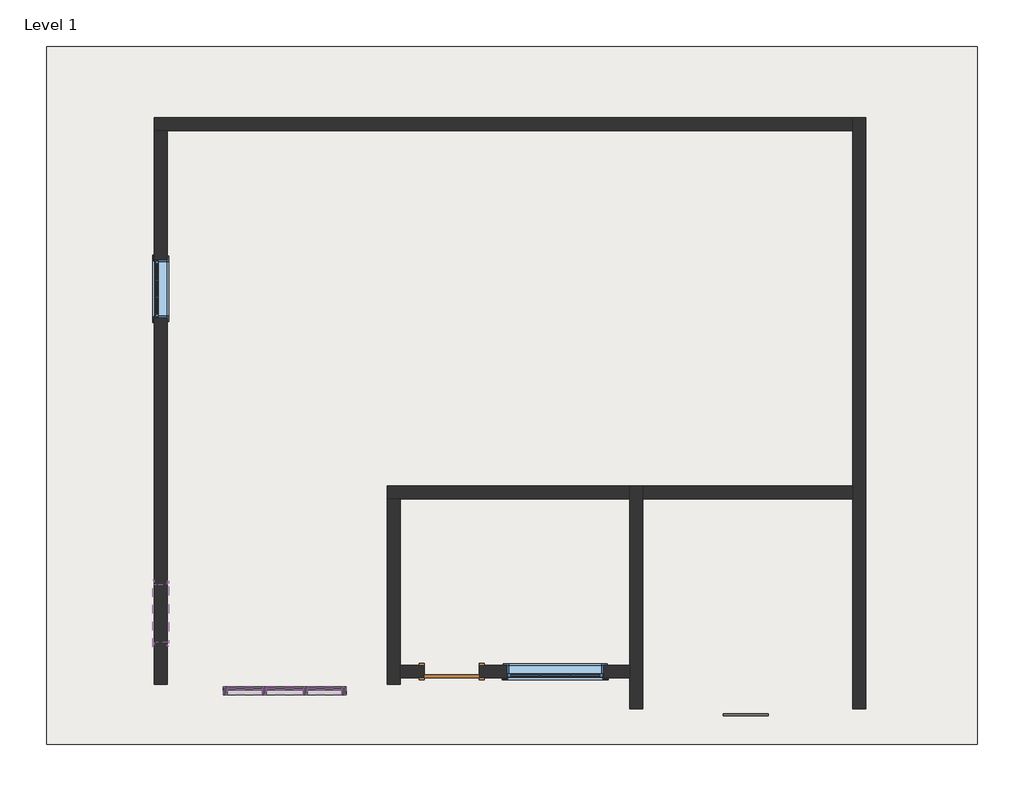
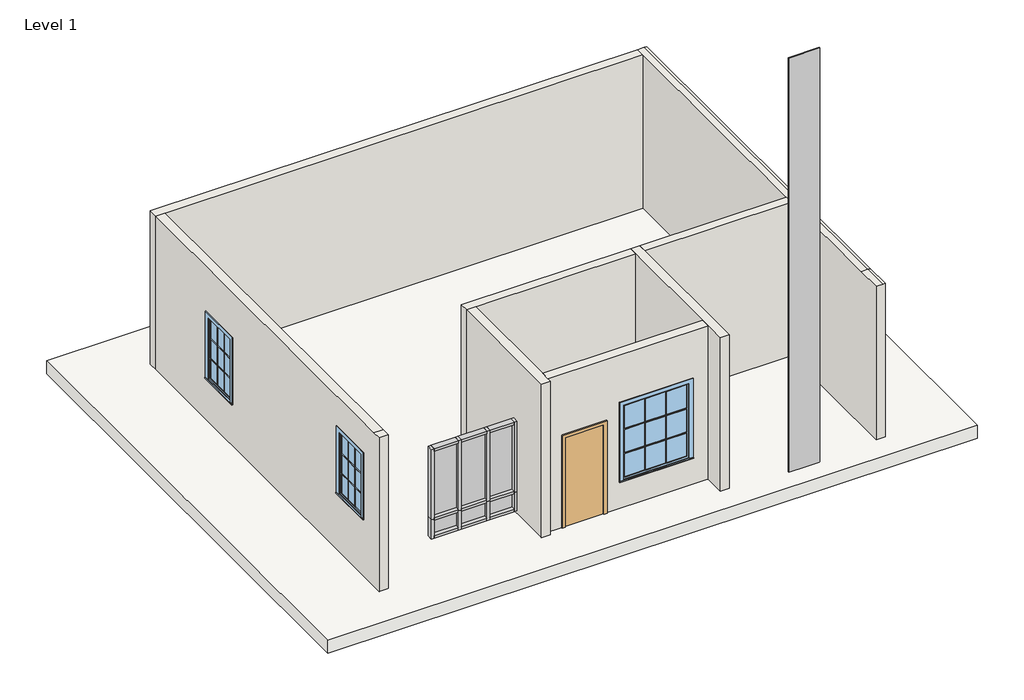
# One storey: 17 members, 8 walls, 7 plates, 3 windows, 1 door, 1 slab.
"""IFC4 building model written with IfcOpenShell, lengths in millimetres."""

from ifc_helpers import new_model, si_unit, frame, origin, origin_with_axes, place, context, project, spatial, polyline, outline, extrude, faceted_brep, transform, mapped, element, save
from components import door_f75d31f8, member_6374d63f, member_ffd4c858, member_912d8bb3, member_c5d18237, member_71656fef, member_15823cb3, member_c78c2eae, member_bdb631d2, system_panel_glazed_05561604, system_panel_glazed_5c6b2ea2, system_panel_glazed_7f181415, system_panel_glazed_51fb9f70, system_panel_glazed_62cbeebf, window_58e1470a, window_f2d3b6b9

model = new_model("IFC4")

# Units and contexts
model_context = context("Model", 3, world=origin())
ifc_project = project(units=[si_unit("LENGTHUNIT", "METRE", prefix="MILLI")], contexts=[model_context])

# Site, building, storey
site = spatial("IfcSite", under=ifc_project)
building = spatial("IfcBuilding", under=site)
storey = spatial("IfcBuildingStorey", under=building, Name="Level 1", Elevation=0.0)

# Door
placement = place(None, origin())
door_shape = door_f75d31f8(model_context)
element("IfcDoor", 1, ObjectType="Single-Flush : 34\" x 84\"", at=placement, inside=storey, context=model_context, shape_type="MappedRepresentation", body=[
    mapped(door_shape, transform((-8075.411895, -370.6574077, 0.0), x_axis=(-1.0, 0.0, 0.0), y_axis=(0.0, -1.0, 0.0), z_axis=(0.0, 0.0, 1.0))),
])

# Members
member_shape = member_6374d63f(model_context)
element("IfcMember", 2, ObjectType="Rectangular Mullion : 2.5\" x 5\" rectangular", at=placement, inside=storey, context=model_context, shape_type="MappedRepresentation", body=[
    mapped(member_shape, transform((-10412.8218023, -675.4574077, 1425.9477294), x_axis=(0.0, 0.0, 1.0), y_axis=(0.0, -1.0, 0.0), z_axis=(1.0, 0.0, 0.0))),
])
member_2_shape = member_ffd4c858(model_context)
element("IfcMember", 3, ObjectType="Rectangular Mullion : 2.5\" x 5\" rectangular", at=placement, inside=storey, context=model_context, shape_type="MappedRepresentation", body=[
    mapped(member_2_shape, transform((-11024.5384689, -675.4574077, 968.7477294), x_axis=(1.0, 0.0, 0.0), y_axis=(0.0, -1.0, 0.0), z_axis=(0.0, 0.0, -1.0))),
])
element("IfcMember", 4, ObjectType="Rectangular Mullion : 2.5\" x 5\" rectangular", at=placement, inside=storey, context=model_context, shape_type="MappedRepresentation", body=[
    mapped(member_2_shape, transform((-10381.0718023, -675.4574077, 968.7477294), x_axis=(1.0, 0.0, 0.0), y_axis=(0.0, -1.0, 0.0), z_axis=(0.0, 0.0, -1.0))),
])
member_3_shape = member_912d8bb3(model_context)
element("IfcMember", 5, ObjectType="Rectangular Mullion : 2.5\" x 5\" rectangular", at=placement, inside=storey, context=model_context, shape_type="MappedRepresentation", body=[
    mapped(member_3_shape, transform((-10992.7884689, -675.4574077, 968.7477294), x_axis=(0.0, 0.0, -1.0), y_axis=(0.0, -1.0, 0.0), z_axis=(-1.0, 0.0, 0.0))),
])
member_4_shape = member_c5d18237(model_context)
element("IfcMember", 6, ObjectType="Rectangular Mullion : 2.5\" x 5\" rectangular", at=placement, inside=storey, context=model_context, shape_type="MappedRepresentation", body=[
    mapped(member_4_shape, transform((-9801.1051356, -675.4574077, 1425.9477294), x_axis=(0.0, 0.0, 1.0), y_axis=(0.0, -1.0, 0.0), z_axis=(1.0, 0.0, 0.0))),
])
element("IfcMember", 7, ObjectType="Rectangular Mullion : 2.5\" x 5\" rectangular", at=placement, inside=storey, context=model_context, shape_type="MappedRepresentation", body=[
    mapped(member_4_shape, transform((-11056.2884689, -675.4574077, 1425.9477294), x_axis=(0.0, 0.0, 1.0), y_axis=(0.0, -1.0, 0.0), z_axis=(1.0, 0.0, 0.0))),
])
member_5_shape = member_71656fef(model_context)
element("IfcMember", 8, ObjectType="Rectangular Mullion : 2.5\" x 5\" rectangular", at=placement, inside=storey, context=model_context, shape_type="MappedRepresentation", body=[
    mapped(member_5_shape, transform((-10349.3218023, -675.4574077, 968.7477294), x_axis=(0.0, 0.0, -1.0), y_axis=(0.0, -1.0, 0.0), z_axis=(-1.0, 0.0, 0.0))),
])
element("IfcMember", 9, ObjectType="Rectangular Mullion : 2.5\" x 5\" rectangular", at=placement, inside=storey, context=model_context, shape_type="MappedRepresentation", body=[
    mapped(member_5_shape, transform((-11604.5051356, -675.4574077, 968.7477294), x_axis=(0.0, 0.0, -1.0), y_axis=(0.0, -1.0, 0.0), z_axis=(-1.0, 0.0, 0.0))),
])
member_6_shape = member_15823cb3(model_context)
element("IfcMember", 10, ObjectType="Rectangular Mullion : 2.5\" x 5\" rectangular", at=placement, inside=storey, context=model_context, shape_type="MappedRepresentation", body=[
    mapped(member_6_shape, transform((-11668.0051356, -675.4574077, 1425.9477294), x_axis=(-1.0, 0.0, 0.0), y_axis=(0.0, -1.0, 0.0), z_axis=(0.0, 0.0, 1.0))),
])
element("IfcMember", 11, ObjectType="Rectangular Mullion : 2.5\" x 5\" rectangular", at=placement, inside=storey, context=model_context, shape_type="MappedRepresentation", body=[
    mapped(member_3_shape, transform((-10412.8218023, -675.4574077, 3102.2835188), x_axis=(0.0, 0.0, 1.0), y_axis=(0.0, -1.0, 0.0), z_axis=(1.0, 0.0, 0.0))),
])
element("IfcMember", 12, ObjectType="Rectangular Mullion : 2.5\" x 5\" rectangular", at=placement, inside=storey, context=model_context, shape_type="MappedRepresentation", body=[
    mapped(member_5_shape, transform((-11056.2884689, -675.4574077, 3102.2835188), x_axis=(0.0, 0.0, 1.0), y_axis=(0.0, -1.0, 0.0), z_axis=(1.0, 0.0, 0.0))),
])
element("IfcMember", 13, ObjectType="Rectangular Mullion : 2.5\" x 5\" rectangular", at=placement, inside=storey, context=model_context, shape_type="MappedRepresentation", body=[
    mapped(member_5_shape, transform((-9801.1051356, -675.4574077, 3102.2835188), x_axis=(0.0, 0.0, 1.0), y_axis=(0.0, -1.0, 0.0), z_axis=(1.0, 0.0, 0.0))),
])
element("IfcMember", 14, ObjectType="Rectangular Mullion : 2.5\" x 5\" rectangular", at=placement, inside=storey, context=model_context, shape_type="MappedRepresentation", body=[
    mapped(member_6_shape, transform((-9737.6051356, -675.4574077, 968.7477294), x_axis=(1.0, 0.0, 0.0), y_axis=(0.0, -1.0, 0.0), z_axis=(0.0, 0.0, -1.0))),
])
member_7_shape = member_c78c2eae(model_context)
element("IfcMember", 15, ObjectType="Rectangular Mullion : 2.5\" x 5\" rectangular", at=placement, inside=storey, context=model_context, shape_type="MappedRepresentation", body=[
    mapped(member_7_shape, transform((-11024.5384689, -675.4574077, 1425.9477294), x_axis=(1.0, 0.0, 0.0), y_axis=(0.0, -1.0, 0.0), z_axis=(0.0, 0.0, -1.0))),
])
element("IfcMember", 16, ObjectType="Rectangular Mullion : 2.5\" x 5\" rectangular", at=placement, inside=storey, context=model_context, shape_type="MappedRepresentation", body=[
    mapped(member_7_shape, transform((-10381.0718023, -675.4574077, 1425.9477294), x_axis=(1.0, 0.0, 0.0), y_axis=(0.0, -1.0, 0.0), z_axis=(0.0, 0.0, -1.0))),
])
member_8_shape = member_bdb631d2(model_context)
element("IfcMember", 17, ObjectType="Rectangular Mullion : 2.5\" x 5\" rectangular", at=placement, inside=storey, context=model_context, shape_type="MappedRepresentation", body=[
    mapped(member_8_shape, transform((-11668.0051356, -675.4574077, 3102.2835188), x_axis=(-1.0, 0.0, 0.0), y_axis=(0.0, -1.0, 0.0), z_axis=(0.0, 0.0, 1.0))),
])
element("IfcMember", 18, ObjectType="Rectangular Mullion : 2.5\" x 5\" rectangular", at=placement, inside=storey, context=model_context, shape_type="MappedRepresentation", body=[
    mapped(member_8_shape, transform((-9737.6051356, -675.4574077, 1425.9477294), x_axis=(1.0, 0.0, 0.0), y_axis=(0.0, -1.0, 0.0), z_axis=(0.0, 0.0, -1.0))),
])

# Plates
system_panel_glazed_shape = system_panel_glazed_05561604(model_context)
element("IfcPlate", 19, ObjectType="System Panel : Glazed", at=placement, inside=storey, context=model_context, shape_type="MappedRepresentation", body=[
    mapped(system_panel_glazed_shape, transform((-3454.524812, -1081.8574077, 0.0), x_axis=(1.0, 0.0, 0.0), y_axis=(0.0, 1.0, 0.0), z_axis=(0.0, 0.0, 1.0))),
])
system_panel_glazed_2_shape = system_panel_glazed_5c6b2ea2(model_context)
element("IfcPlate", 20, ObjectType="System Panel : Glazed", at=placement, inside=storey, context=model_context, shape_type="MappedRepresentation", body=[
    mapped(system_panel_glazed_2_shape, transform((-10702.8051356, -675.4574077, 1032.2477294), x_axis=(1.0, 0.0, 0.0), y_axis=(0.0, 1.0, 0.0), z_axis=(0.0, 0.0, 1.0))),
])
system_panel_glazed_3_shape = system_panel_glazed_7f181415(model_context)
element("IfcPlate", 21, ObjectType="System Panel : Glazed", at=placement, inside=storey, context=model_context, shape_type="MappedRepresentation", body=[
    mapped(system_panel_glazed_3_shape, transform((-11330.3968023, -675.4574077, 1032.2477294), x_axis=(1.0, 0.0, 0.0), y_axis=(0.0, 1.0, 0.0), z_axis=(0.0, 0.0, 1.0))),
])
element("IfcPlate", 22, ObjectType="System Panel : Glazed", at=placement, inside=storey, context=model_context, shape_type="MappedRepresentation", body=[
    mapped(system_panel_glazed_3_shape, transform((-10075.2134689, -675.4574077, 1032.2477294), x_axis=(1.0, 0.0, 0.0), y_axis=(0.0, 1.0, 0.0), z_axis=(0.0, 0.0, 1.0))),
])
system_panel_glazed_4_shape = system_panel_glazed_51fb9f70(model_context)
element("IfcPlate", 23, ObjectType="System Panel : Glazed", at=placement, inside=storey, context=model_context, shape_type="MappedRepresentation", body=[
    mapped(system_panel_glazed_4_shape, transform((-10702.8051356, -675.4574077, 1457.6977294), x_axis=(1.0, 0.0, 0.0), y_axis=(0.0, 1.0, 0.0), z_axis=(0.0, 0.0, 1.0))),
])
system_panel_glazed_5_shape = system_panel_glazed_62cbeebf(model_context)
element("IfcPlate", 24, ObjectType="System Panel : Glazed", at=placement, inside=storey, context=model_context, shape_type="MappedRepresentation", body=[
    mapped(system_panel_glazed_5_shape, transform((-11330.3968023, -675.4574077, 1457.6977294), x_axis=(1.0, 0.0, 0.0), y_axis=(0.0, 1.0, 0.0), z_axis=(0.0, 0.0, 1.0))),
])
element("IfcPlate", 25, ObjectType="System Panel : Glazed", at=placement, inside=storey, context=model_context, shape_type="MappedRepresentation", body=[
    mapped(system_panel_glazed_5_shape, transform((-10075.2134689, -675.4574077, 1457.6977294), x_axis=(1.0, 0.0, 0.0), y_axis=(0.0, 1.0, 0.0), z_axis=(0.0, 0.0, 1.0))),
])

# Slab
element("IfcSlab", 26, ObjectType="Generic - 12\"", at=placement, inside=storey, context=model_context, shape_type="SweptSolid", body=[
    extrude(outline(polyline([(185.9133397, 9459.386183), (185.9133397, -1513.413817), (-14444.4866603, -1513.413817), (-14444.4866603, 9459.386183), (185.9133397, 9459.386183)])), frame((0.0, 0.0, -304.8), z_axis=(0.0, 0.0, 1.0), x_axis=(1.0, 0.0, 0.0)), (0.0, 0.0, 1.0), 304.8),
])

# Walls
element("IfcWall", 27, ObjectType="Generic - 8\"", at=placement, inside=storey, context=model_context, shape_type="Brep", body=[
    faceted_brep([(-12749.011895, 8138.3425923, 0.0), (-12545.811895, 8138.3425923, 0.0), (-1776.211895, 8138.3425923, 0.0), (-1776.211895, 8138.3425923, 3657.6), (-12545.811895, 8138.3425923, 3657.6), (-12749.011895, 8138.3425923, 3657.6), (-12749.011895, 8341.5425923, 0.0), (-12749.011895, 8341.5425923, 3657.6), (-1776.211895, 8341.5425923, 3657.6), (-1776.211895, 8341.5425923, 0.0)], [[[0, 1, 2, 3, 4, 5]], [[6, 7, 8, 9]], [[2, 1, 0, 6, 9]], [[0, 5, 7, 6]], [[3, 2, 9, 8]], [[5, 4, 3, 8, 7]]]),
])
element("IfcWall", 28, ObjectType="Generic - 8\"", at=placement, inside=storey, context=model_context, shape_type="SweptSolid", body=[
    extrude(outline(polyline([(-573.8574077, 0.0), (-573.8574077, 3657.6), (-377.2618819, 3657.6), (8138.3425923, 3657.6), (8138.3425923, 0.0), (-573.8574077, 0.0)]), holes=[polyline([(6106.3425923, 2518.3948207), (5191.9425923, 2518.3948207), (5191.9425923, 994.3948207), (6106.3425923, 994.3948207), (6106.3425923, 2518.3948207)]), polyline([(1000.9425923, 2880.0484456), (86.5425923, 2880.0484456), (86.5425923, 1356.0484456), (1000.9425923, 1356.0484456), (1000.9425923, 2880.0484456)])]), frame((-12749.011895, 0.0, 0.0), z_axis=(1.0, 0.0, 0.0), x_axis=(0.0, 1.0, 0.0)), (0.0, 0.0, 1.0), 203.2),
])
element("IfcWall", 29, ObjectType="Generic - 8\"", at=placement, inside=storey, context=model_context, shape_type="Brep", body=[
    faceted_brep([(-1776.211895, 8341.5425923, 0.0), (-1776.211895, 8138.3425923, 0.0), (-1776.211895, 2550.3425923, 0.0), (-1776.211895, 2347.1425923, 0.0), (-1776.211895, -954.8574077, 0.0), (-1776.211895, -954.8574077, 3657.6), (-1776.211895, -377.0074077, 3657.6), (-1776.211895, 2347.1425923, 3657.6), (-1776.211895, 2448.7425923, 3657.6), (-1776.211895, 2550.3425923, 3657.6), (-1776.211895, 8138.3425923, 3657.6), (-1776.211895, 8341.5425923, 3657.6), (-1573.011895, 8341.5425923, 0.0), (-1573.011895, 8341.5425923, 3657.6), (-1573.011895, 2448.7425923, 3657.6), (-1573.011895, -377.0074077, 3657.6), (-1573.011895, -954.8574077, 3657.6), (-1573.011895, -954.8574077, 0.0), (-1623.5722278, 8341.5425923, 3657.6), (-1623.5722278, -954.8574077, 3657.6), (-1623.5722278, -377.0074077, 3657.6)], [[[0, 1, 2, 3, 4, 5, 6, 7, 8, 9, 10, 11]], [[12, 13, 14, 15, 16, 17]], [[4, 3, 2, 1, 0, 12, 17]], [[0, 11, 18, 13, 12]], [[6, 5, 19, 20]], [[15, 14, 13, 18, 20]], [[19, 16, 15, 20]], [[11, 10, 9, 8, 7, 6, 20, 18]], [[5, 4, 17, 16, 19]]]),
])
element("IfcWall", 30, ObjectType="Generic - 8\"", at=placement, inside=storey, context=model_context, shape_type="Brep", body=[
    faceted_brep([(-5078.211895, -954.8574077, 0.0), (-5078.211895, 2347.1425923, 0.0), (-5078.211895, 2550.3425923, 0.0), (-5078.211895, 2550.3425923, 3657.6), (-5078.211895, 2347.1425923, 3657.6), (-5078.211895, -954.8574077, 3657.6), (-5281.411895, -954.8574077, 0.0), (-5281.411895, -954.8574077, 3657.6), (-5281.411895, -472.2574077, 3657.6), (-5281.411895, -269.0574077, 3657.6), (-5281.411895, 2347.1425923, 3657.6), (-5281.411895, 2550.3425923, 3657.6), (-5281.411895, 2550.3425923, 0.0), (-5281.411895, 2347.1425923, 0.0), (-5281.411895, -269.0574077, 0.0), (-5281.411895, -472.2574077, 0.0)], [[[0, 1, 2, 3, 4, 5]], [[6, 7, 8, 9, 10, 11, 12, 13, 14, 15]], [[2, 1, 0, 6, 15, 14, 13, 12]], [[5, 4, 3, 11, 10, 9, 8, 7]], [[0, 5, 7, 6]], [[3, 2, 12, 11]]]),
])
element("IfcWall", 31, ObjectType="Generic - 8\"", at=placement, inside=storey, context=model_context, shape_type="SweptSolid", body=[
    extrude(outline(polyline([(-1776.211895, 2347.1425923), (-5078.211895, 2347.1425923), (-5078.211895, 2550.3425923), (-1776.211895, 2550.3425923), (-1776.211895, 2347.1425923)])), origin_with_axes(), (0.0, 0.0, 1.0), 3657.6),
])
element("IfcWall", 32, ObjectType="Generic - 8\"", at=placement, inside=storey, context=model_context, shape_type="Brep", body=[
    faceted_brep([(-5281.411895, 2550.3425923, 0.0), (-9091.411895, 2550.3425923, 0.0), (-9091.411895, 2550.3425923, 3657.6), (-5281.411895, 2550.3425923, 3657.6), (-5281.411895, 2347.1425923, 0.0), (-5281.411895, 2347.1425923, 3657.6), (-8888.211895, 2347.1425923, 3657.6), (-9091.411895, 2347.1425923, 3657.6), (-9091.411895, 2347.1425923, 0.0), (-8888.211895, 2347.1425923, 0.0)], [[[0, 1, 2, 3]], [[4, 5, 6, 7, 8, 9]], [[1, 0, 4, 9, 8]], [[3, 2, 7, 6, 5]], [[0, 3, 5, 4]], [[2, 1, 8, 7]]]),
])
element("IfcWall", 33, ObjectType="Generic - 8\"", at=placement, inside=storey, context=model_context, shape_type="Brep", body=[
    faceted_brep([(-9091.411895, 2347.1425923, 0.0), (-9091.411895, -573.8574077, 0.0), (-9091.411895, -573.8574077, 3657.6), (-9091.411895, 2347.1425923, 3657.6), (-8888.211895, 2347.1425923, 0.0), (-8888.211895, 2347.1425923, 3657.6), (-8888.211895, -269.0574077, 3657.6), (-8888.211895, -472.2574077, 3657.6), (-8888.211895, -573.8574077, 3657.6), (-8888.211895, -573.8574077, 0.0), (-8888.211895, -472.2574077, 0.0), (-8888.211895, -269.0574077, 0.0)], [[[0, 1, 2, 3]], [[4, 5, 6, 7, 8, 9, 10, 11]], [[1, 0, 4, 11, 10, 9]], [[3, 2, 8, 7, 6, 5]], [[0, 3, 5, 4]], [[2, 1, 9, 8]]]),
])
element("IfcWall", 34, ObjectType="Generic - 8\"", at=placement, inside=storey, context=model_context, shape_type="SweptSolid", body=[
    extrude(outline(polyline([(0.0, -8888.211895), (0.0, -8507.211895), (2133.6, -8507.211895), (2133.6, -7643.611895), (0.0, -7643.611895), (0.0, -5281.411895), (3657.6, -5281.411895), (3657.6, -8888.211895), (0.0, -8888.211895)]), holes=[polyline([(2458.4976404, -7211.811895), (2458.4976404, -5687.811895), (629.6976404, -5687.811895), (629.6976404, -7211.811895), (2458.4976404, -7211.811895)])]), frame((0.0, -472.2574077, 0.0), z_axis=(0.0, 1.0, 0.0), x_axis=(0.0, 0.0, 1.0)), (0.0, 0.0, 1.0), 203.2),
])

# Windows
window_shape = window_58e1470a(model_context)
element("IfcWindow", 35, ObjectType="Casement 3x3 with Trim : 36\" x 60\"", at=placement, inside=storey, context=model_context, shape_type="MappedRepresentation", body=[
    mapped(window_shape, transform((-12647.411895, 5649.1425923, 384.7948207), x_axis=(0.0, 1.0, 0.0), y_axis=(-1.0, 0.0, 0.0), z_axis=(0.0, 0.0, 1.0))),
])
element("IfcWindow", 36, ObjectType="Casement 3x3 with Trim : 36\" x 60\"", at=placement, inside=storey, context=model_context, shape_type="MappedRepresentation", body=[
    mapped(window_shape, transform((-12647.411895, 543.7425923, 746.4484456), x_axis=(0.0, 1.0, 0.0), y_axis=(-1.0, 0.0, 0.0), z_axis=(0.0, 0.0, 1.0))),
])
window_2_shape = window_f2d3b6b9(model_context)
element("IfcWindow", 37, ObjectType="Casement 3x3 with Trim : 60\" x 72\"", at=placement, inside=storey, context=model_context, shape_type="MappedRepresentation", body=[
    mapped(window_2_shape, transform((-6449.811895, -370.6574077, -284.7023596), x_axis=(-1.0, 0.0, 0.0), y_axis=(0.0, -1.0, 0.0), z_axis=(0.0, 0.0, 1.0))),
])

save(model, "model.ifc")

# Revit data of these elements
# Type "Single-Flush : 34\" x 84\""
#   Type Mark = "2"
#   Construction Type Id = "MDOOR"
#   Assembly Code = "C1020"
#   Analytic Construction = "Metal"
#   Thickness = 0' - 2"
#   Heat Transfer Coefficient (U) = 0.651978 BTU/(h·ft²·°F)
#   Height = 7' - 0"
#   Trim Projection Ext = 0' - 1"
#   Trim Projection Int = 0' - 1"
#   Trim Width = 0' - 3"
#   Width = 2' - 10"
#   Define Thermal Properties by = 1
#   Door Material = Door - Panel
#   Frame Material = Door - Frame
#   Visual Light Transmittance = 0
#   Solar Heat Gain Coefficient = 0
#   Function = (empty or 0)
#   Wall Closure = (empty or 0)
# Type "Rectangular Mullion : 2.5\" x 5\" rectangular"
#   built-in parameter 1007304 = 0.416667 (stored number, unit not read)
#   built-in parameter 1007301 = 0.104167 (stored number, unit not read)
#   built-in parameter 1007300 = 0.104167 (stored number, unit not read)
# Type "System Panel : Glazed"
#   Construction Type Id = "GSP4R"
#   Analytic Construction = "1/8 in Pilkington single glazing"
#   Visual Light Transmittance = 0.9
#   Solar Heat Gain Coefficient = 0.86
#   Heat Transfer Coefficient (U) = 1.18115 BTU/(h·ft²·°F)
# Type "Generic - 12\""
#   Assembly Code = "B1010"
#   Function = 0
#   Layers, outside or top first: 1' - 0" no material (function 1)
# Type "Generic - 8\""
#   Assembly Code = "B2010"
#   Layers, outside or top first: 0' - 8" no material (function 1)
# Type "Casement 3x3 with Trim : 36\" x 60\""
#   Type Mark = "11"
#   Construction Type Id = "GSP4R"
#   Assembly Code = "B2020100"
#   Analytic Construction = "1/8 in Pilkington single glazing"
#   Visual Light Transmittance = 0.9
#   Solar Heat Gain Coefficient = 0.78
#   Heat Transfer Coefficient (U) = 0.6496 BTU/(h·ft²·°F)
#   Height = 5' - 0"
#   Default Sill Height = 2' - 0"
#   Trim Projection - Ext. = 0' - 0 1/2"
#   Trim Projection - Int. = 0' - 0 3/4"
#   Trim Width - Exterior = 0' - 3 1/2"
#   Trim Width - Interior = 0' - 3 1/2"
#   Width = 3' - 0"
#   Window Inset = 0' - 0 3/4"
#   Define Thermal Properties by = 1
#   Glass Pane Material = Glass
#   Sash Material = Sash
#   Trim Exterior Material = Trim
#   Trim Interior Material = Trim
#   Wall Closure = (empty or 0)
# Type "Casement 3x3 with Trim : 60\" x 72\""
#   Type Mark = "10"
#   Construction Type Id = "GSP4R"
#   Assembly Code = "B2020100"
#   Analytic Construction = "1/8 in Pilkington single glazing"
#   Visual Light Transmittance = 0.9
#   Solar Heat Gain Coefficient = 0.78
#   Heat Transfer Coefficient (U) = 0.6496 BTU/(h·ft²·°F)
#   Height = 6' - 0"
#   Default Sill Height = 3' - 0"
#   Trim Projection - Ext. = 0' - 0 1/2"
#   Trim Projection - Int. = 0' - 0 3/4"
#   Trim Width - Exterior = 0' - 3 1/2"
#   Trim Width - Interior = 0' - 3 1/2"
#   Width = 5' - 0"
#   Window Inset = 0' - 0 3/4"
#   Define Thermal Properties by = 1
#   Glass Pane Material = Glass
#   Sash Material = Sash
#   Trim Exterior Material = Trim
#   Trim Interior Material = Trim
#   Wall Closure = (empty or 0)
# Element 1 (IfcDoor, "Single-Flush : 34\" x 84\"")
#   Phase Created = New Construction
#   Materials on its faces: "Door - Frame", "Door - Panel"
# Elements 2, 3, 4, 5, 6, 7, 8, 9, 10, 11, 12, 13, 14, 15, 16, 17, 18 (IfcMember, "Rectangular Mullion : 2.5\" x 5\" rectangular")
#   Phase Created = New Construction
#   Materials on its faces: "Aluminum"
# Elements 19, 20, 21, 22, 23, 24, 25 (IfcPlate, "System Panel : Glazed")
#   Phase Created = New Construction
#   Materials on its faces: "Glass"
# Element 26 (IfcSlab, "Generic - 12\"")
#   Height Offset From Level = 0' - 0"
#   Phase Created = New Construction
#   Materials on its faces: "Default Floor"
# Elements 27, 28, 29, 30, 31, 32, 33, 34 (IfcWall, "Generic - 8\"")
#   Top Offset = 0' - 0"
#   Base Offset = 0' - 0"
#   Unconnected Height = 12' - 0"
#   wall height = 12' - 0"
#   Phase Created = New Construction
#   Base Constraint = Level 1
#   Materials on its faces: "Default Wall"
# Element 35 (IfcWindow, "Casement 3x3 with Trim : 36\" x 60\"")
#   Mark = "3"
#   Phase Created = New Construction
#   Materials on its faces: "Sash", "Glass", "Trim"
# Element 36 (IfcWindow, "Casement 3x3 with Trim : 36\" x 60\"")
#   Mark = "4"
#   Phase Created = New Construction
#   Materials on its faces: "Sash", "Glass", "Trim"
# Element 37 (IfcWindow, "Casement 3x3 with Trim : 60\" x 72\"")
#   Mark = "1"
#   Phase Created = New Construction
#   Materials on its faces: "Sash", "Glass", "Trim"
# Materials
#   "Door - Panel": class "Wood", colour RGB 210 159 95, transparency 0
#   "Door - Frame": colour RGB 118 70 51, transparency 0
#   "Glass": class "Glass", colour RGB 0 128 192, transparency 0.75, Description = "Soda Lime Glass", Cost = 0
#   "Sash": class "Wood", colour RGB 224 178 126, transparency 0
#   "Trim": class "Wood", colour RGB 224 178 126, transparency 0
#   "Aluminum": class "Metal", colour RGB 247 247 247, transparency 0, Description = "Aluminum 6061", Cost = 0
#   "Default Floor": colour RGB 128 128 128, transparency 0
#   "Default Wall": colour RGB 128 128 128, transparency 0
